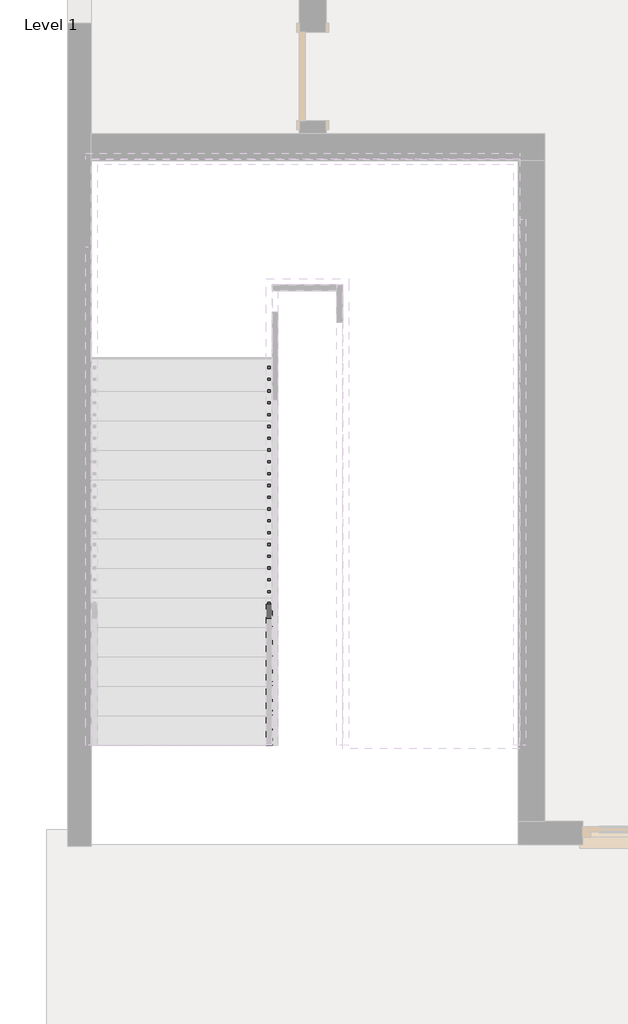
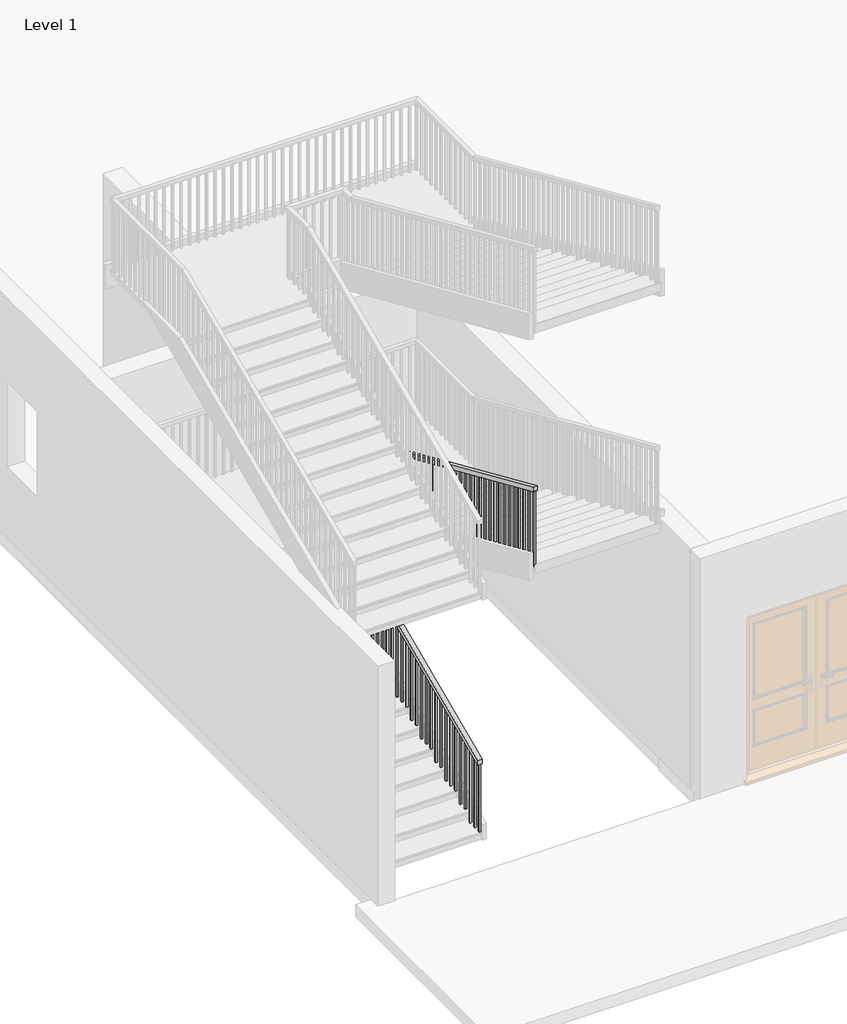
# One storey, part 2 of 6: 1 railing.
"""IFC4 building model written with IfcOpenShell, lengths in millimetres."""

from ifc_helpers import new_model, si_unit, frame, origin, place, context, project, spatial, polyline, outline, extrude, faceted_brep, element, save

model = new_model("IFC4")

# Units and contexts
model_context = context("Model", 3, world=origin())
ifc_project = project(units=[si_unit("LENGTHUNIT", "METRE", prefix="MILLI")], contexts=[model_context])

# Site, building, storey
site = spatial("IfcSite", under=ifc_project)
building = spatial("IfcBuilding", under=site)
storey = spatial("IfcBuildingStorey", under=building, Name="Level 1", Elevation=0.0)

# Railing
placement = place(None, origin())
element("IfcRailing", 1, ObjectType="Handrail - Rectangular", at=placement, inside=storey, context=model_context, shape_type="SolidModel", body=[
    faceted_brep([(-6050.7290366, -6973.0610642, 721.36), (-6050.7290366, -6973.0610642, 665.8599828), (-5999.9290366, -6973.0610642, 665.8599828), (-5999.9290366, -6973.0610642, 721.36), (-6050.7290366, -3417.0610642, 2286.0), (-6050.7290366, -3406.3792071, 2235.2), (-5999.9290366, -3406.3792071, 2235.2), (-5999.9290366, -3417.0610642, 2286.0), (-6050.7290366, -2959.8610642, 2286.0), (-6050.7290366, -2959.8610642, 2235.2), (-5999.9290366, -3010.6610642, 2235.2), (-5999.9290366, -3010.6610642, 2286.0), (-5339.5290366, -2959.8610642, 2286.0), (-5339.5290366, -2959.8610642, 2235.2), (-5390.3290366, -3010.6610642, 2235.2), (-5390.3290366, -3010.6610642, 2286.0), (-5339.5290366, -3163.0610642, 2286.0), (-5339.5290366, -3173.7429214, 2235.2), (-5390.3290366, -3173.7429214, 2235.2), (-5390.3290366, -3163.0610642, 2286.0), (-5339.5290366, -6973.0610642, 3962.4), (-5390.3290366, -6973.0610642, 3962.4), (-5390.3290366, -6973.0610642, 3906.8999828), (-5339.5290366, -6973.0610642, 3906.8999828)], [[[0, 1, 2, 3]], [[1, 0, 4, 5]], [[2, 1, 5, 6]], [[3, 2, 6, 7]], [[0, 3, 7, 4]], [[5, 4, 8, 9]], [[6, 5, 9, 10]], [[7, 6, 10, 11]], [[4, 7, 11, 8]], [[9, 8, 12, 13]], [[10, 9, 13, 14]], [[11, 10, 14, 15]], [[8, 11, 15, 12]], [[13, 12, 16, 17]], [[14, 13, 17, 18]], [[15, 14, 18, 19]], [[12, 15, 19, 16]], [[20, 21, 22, 23]], [[17, 16, 20, 23]], [[18, 17, 23, 22]], [[19, 18, 22, 21]], [[16, 19, 21, 20]]]),
    extrude(outline(polyline([(-6957.1860642, 3899.9149828), (-6938.1360642, 3891.5329828), (-6938.1360642, 2936.24), (-6957.1860642, 2936.24), (-6957.1860642, 3899.9149828)])), frame((-5374.4540366, 0.0, 0.0), z_axis=(1.0, 0.0, 0.0), x_axis=(0.0, 1.0, 0.0)), (0.0, 0.0, 1.0), 19.05),
    extrude(outline(polyline([(-6855.5860642, 3855.2109828), (-6836.5360642, 3846.8289828), (-6836.5360642, 2936.24), (-6855.5860642, 2936.24), (-6855.5860642, 3855.2109828)])), frame((-5374.4540366, 0.0, 0.0), z_axis=(1.0, 0.0, 0.0), x_axis=(0.0, 1.0, 0.0)), (0.0, 0.0, 1.0), 19.05),
    extrude(outline(polyline([(-6753.9860642, 3810.5069828), (-6734.9360642, 3802.1249828), (-6734.9360642, 2936.24), (-6753.9860642, 2936.24), (-6753.9860642, 3810.5069828)])), frame((-5374.4540366, 0.0, 0.0), z_axis=(1.0, 0.0, 0.0), x_axis=(0.0, 1.0, 0.0)), (0.0, 0.0, 1.0), 19.05),
    extrude(outline(polyline([(-6652.3860642, 3765.8029828), (-6633.3360642, 3757.4209828), (-6633.3360642, 2824.48), (-6652.3860642, 2824.48), (-6652.3860642, 3765.8029828)])), frame((-5374.4540366, 0.0, 0.0), z_axis=(1.0, 0.0, 0.0), x_axis=(0.0, 1.0, 0.0)), (0.0, 0.0, 1.0), 19.05),
    extrude(outline(polyline([(-6550.7860642, 3721.0989828), (-6531.7360642, 3712.7169828), (-6531.7360642, 2824.48), (-6550.7860642, 2824.48), (-6550.7860642, 3721.0989828)])), frame((-5374.4540366, 0.0, 0.0), z_axis=(1.0, 0.0, 0.0), x_axis=(0.0, 1.0, 0.0)), (0.0, 0.0, 1.0), 19.05),
    extrude(outline(polyline([(-6449.1860642, 3676.3949828), (-6430.1360642, 3668.0129828), (-6430.1360642, 2712.72), (-6449.1860642, 2712.72), (-6449.1860642, 3676.3949828)])), frame((-5374.4540366, 0.0, 0.0), z_axis=(1.0, 0.0, 0.0), x_axis=(0.0, 1.0, 0.0)), (0.0, 0.0, 1.0), 19.05),
    extrude(outline(polyline([(-6347.5860642, 3631.6909828), (-6328.5360642, 3623.3089828), (-6328.5360642, 2712.72), (-6347.5860642, 2712.72), (-6347.5860642, 3631.6909828)])), frame((-5374.4540366, 0.0, 0.0), z_axis=(1.0, 0.0, 0.0), x_axis=(0.0, 1.0, 0.0)), (0.0, 0.0, 1.0), 19.05),
    extrude(outline(polyline([(-6245.9860642, 3586.9869828), (-6226.9360642, 3578.6049828), (-6226.9360642, 2712.72), (-6245.9860642, 2712.72), (-6245.9860642, 3586.9869828)])), frame((-5374.4540366, 0.0, 0.0), z_axis=(1.0, 0.0, 0.0), x_axis=(0.0, 1.0, 0.0)), (0.0, 0.0, 1.0), 19.05),
    extrude(outline(polyline([(-6144.3860642, 3542.2829828), (-6125.3360642, 3533.9009828), (-6125.3360642, 2600.96), (-6144.3860642, 2600.96), (-6144.3860642, 3542.2829828)])), frame((-5374.4540366, 0.0, 0.0), z_axis=(1.0, 0.0, 0.0), x_axis=(0.0, 1.0, 0.0)), (0.0, 0.0, 1.0), 19.05),
    extrude(outline(polyline([(-6042.7860642, 3497.5789828), (-6023.7360642, 3489.1969828), (-6023.7360642, 2600.96), (-6042.7860642, 2600.96), (-6042.7860642, 3497.5789828)])), frame((-5374.4540366, 0.0, 0.0), z_axis=(1.0, 0.0, 0.0), x_axis=(0.0, 1.0, 0.0)), (0.0, 0.0, 1.0), 19.05),
    extrude(outline(polyline([(-5941.1860642, 3452.8749828), (-5922.1360642, 3444.4929828), (-5922.1360642, 2489.2), (-5941.1860642, 2489.2), (-5941.1860642, 3452.8749828)])), frame((-5374.4540366, 0.0, 0.0), z_axis=(1.0, 0.0, 0.0), x_axis=(0.0, 1.0, 0.0)), (0.0, 0.0, 1.0), 19.05),
    extrude(outline(polyline([(-5839.5860642, 3408.1709828), (-5820.5360642, 3399.7889828), (-5820.5360642, 2489.2), (-5839.5860642, 2489.2), (-5839.5860642, 3408.1709828)])), frame((-5374.4540366, 0.0, 0.0), z_axis=(1.0, 0.0, 0.0), x_axis=(0.0, 1.0, 0.0)), (0.0, 0.0, 1.0), 19.05),
    extrude(outline(polyline([(-5737.9860642, 3363.4669828), (-5718.9360642, 3355.0849828), (-5718.9360642, 2489.2), (-5737.9860642, 2489.2), (-5737.9860642, 3363.4669828)])), frame((-5374.4540366, 0.0, 0.0), z_axis=(1.0, 0.0, 0.0), x_axis=(0.0, 1.0, 0.0)), (0.0, 0.0, 1.0), 19.05),
    extrude(outline(polyline([(-5636.3860642, 3318.7629828), (-5617.3360642, 3310.3809828), (-5617.3360642, 2377.44), (-5636.3860642, 2377.44), (-5636.3860642, 3318.7629828)])), frame((-5374.4540366, 0.0, 0.0), z_axis=(1.0, 0.0, 0.0), x_axis=(0.0, 1.0, 0.0)), (0.0, 0.0, 1.0), 19.05),
    extrude(outline(polyline([(-5534.7860642, 3274.0589828), (-5515.7360642, 3265.6769828), (-5515.7360642, 2377.44), (-5534.7860642, 2377.44), (-5534.7860642, 3274.0589828)])), frame((-5374.4540366, 0.0, 0.0), z_axis=(1.0, 0.0, 0.0), x_axis=(0.0, 1.0, 0.0)), (0.0, 0.0, 1.0), 19.05),
    extrude(outline(polyline([(-5433.1860642, 3229.3549828), (-5414.1360642, 3220.9729828), (-5414.1360642, 2265.68), (-5433.1860642, 2265.68), (-5433.1860642, 3229.3549828)])), frame((-5374.4540366, 0.0, 0.0), z_axis=(1.0, 0.0, 0.0), x_axis=(0.0, 1.0, 0.0)), (0.0, 0.0, 1.0), 19.05),
    extrude(outline(polyline([(-5331.5860642, 3184.6509828), (-5312.5360642, 3176.2689828), (-5312.5360642, 2265.68), (-5331.5860642, 2265.68), (-5331.5860642, 3184.6509828)])), frame((-5374.4540366, 0.0, 0.0), z_axis=(1.0, 0.0, 0.0), x_axis=(0.0, 1.0, 0.0)), (0.0, 0.0, 1.0), 19.05),
    extrude(outline(polyline([(-5229.9860642, 3139.9469828), (-5210.9360642, 3131.5649828), (-5210.9360642, 2265.68), (-5229.9860642, 2265.68), (-5229.9860642, 3139.9469828)])), frame((-5374.4540366, 0.0, 0.0), z_axis=(1.0, 0.0, 0.0), x_axis=(0.0, 1.0, 0.0)), (0.0, 0.0, 1.0), 19.05),
    extrude(outline(polyline([(-5128.3860642, 3095.2429828), (-5109.3360642, 3086.8609828), (-5109.3360642, 2153.92), (-5128.3860642, 2153.92), (-5128.3860642, 3095.2429828)])), frame((-5374.4540366, 0.0, 0.0), z_axis=(1.0, 0.0, 0.0), x_axis=(0.0, 1.0, 0.0)), (0.0, 0.0, 1.0), 19.05),
    extrude(outline(polyline([(-5026.7860642, 3050.5389828), (-5007.7360642, 3042.1569828), (-5007.7360642, 2153.92), (-5026.7860642, 2153.92), (-5026.7860642, 3050.5389828)])), frame((-5374.4540366, 0.0, 0.0), z_axis=(1.0, 0.0, 0.0), x_axis=(0.0, 1.0, 0.0)), (0.0, 0.0, 1.0), 19.05),
    extrude(outline(polyline([(-4925.1860642, 3005.8349828), (-4906.1360642, 2997.4529828), (-4906.1360642, 2042.16), (-4925.1860642, 2042.16), (-4925.1860642, 3005.8349828)])), frame((-5374.4540366, 0.0, 0.0), z_axis=(1.0, 0.0, 0.0), x_axis=(0.0, 1.0, 0.0)), (0.0, 0.0, 1.0), 19.05),
    extrude(outline(polyline([(-4823.5860642, 2961.1309828), (-4804.5360642, 2952.7489828), (-4804.5360642, 2042.16), (-4823.5860642, 2042.16), (-4823.5860642, 2961.1309828)])), frame((-5374.4540366, 0.0, 0.0), z_axis=(1.0, 0.0, 0.0), x_axis=(0.0, 1.0, 0.0)), (0.0, 0.0, 1.0), 19.05),
    extrude(outline(polyline([(-4721.9860642, 2916.4269828), (-4702.9360642, 2908.0449828), (-4702.9360642, 2042.16), (-4721.9860642, 2042.16), (-4721.9860642, 2916.4269828)])), frame((-5374.4540366, 0.0, 0.0), z_axis=(1.0, 0.0, 0.0), x_axis=(0.0, 1.0, 0.0)), (0.0, 0.0, 1.0), 19.05),
    extrude(outline(polyline([(-4620.3860642, 2871.7229828), (-4601.3360642, 2863.3409828), (-4601.3360642, 1930.4), (-4620.3860642, 1930.4), (-4620.3860642, 2871.7229828)])), frame((-5374.4540366, 0.0, 0.0), z_axis=(1.0, 0.0, 0.0), x_axis=(0.0, 1.0, 0.0)), (0.0, 0.0, 1.0), 19.05),
    extrude(outline(polyline([(-4518.7860642, 2827.0189828), (-4499.7360642, 2818.6369828), (-4499.7360642, 1930.4), (-4518.7860642, 1930.4), (-4518.7860642, 2827.0189828)])), frame((-5374.4540366, 0.0, 0.0), z_axis=(1.0, 0.0, 0.0), x_axis=(0.0, 1.0, 0.0)), (0.0, 0.0, 1.0), 19.05),
    extrude(outline(polyline([(-4417.1860642, 2782.3149828), (-4398.1360642, 2773.9329828), (-4398.1360642, 1818.64), (-4417.1860642, 1818.64), (-4417.1860642, 2782.3149828)])), frame((-5374.4540366, 0.0, 0.0), z_axis=(1.0, 0.0, 0.0), x_axis=(0.0, 1.0, 0.0)), (0.0, 0.0, 1.0), 19.05),
    extrude(outline(polyline([(-4315.5860642, 2737.6109828), (-4296.5360642, 2729.2289828), (-4296.5360642, 1818.64), (-4315.5860642, 1818.64), (-4315.5860642, 2737.6109828)])), frame((-5374.4540366, 0.0, 0.0), z_axis=(1.0, 0.0, 0.0), x_axis=(0.0, 1.0, 0.0)), (0.0, 0.0, 1.0), 19.05),
    extrude(outline(polyline([(-4213.9860642, 2692.9069828), (-4194.9360642, 2684.5249828), (-4194.9360642, 1818.64), (-4213.9860642, 1818.64), (-4213.9860642, 2692.9069828)])), frame((-5374.4540366, 0.0, 0.0), z_axis=(1.0, 0.0, 0.0), x_axis=(0.0, 1.0, 0.0)), (0.0, 0.0, 1.0), 19.05),
    extrude(outline(polyline([(-4112.3860642, 2648.2029828), (-4093.3360642, 2639.8209828), (-4093.3360642, 1706.88), (-4112.3860642, 1706.88), (-4112.3860642, 2648.2029828)])), frame((-5374.4540366, 0.0, 0.0), z_axis=(1.0, 0.0, 0.0), x_axis=(0.0, 1.0, 0.0)), (0.0, 0.0, 1.0), 19.05),
    extrude(outline(polyline([(-4010.7860642, 2603.4989828), (-3991.7360642, 2595.1169828), (-3991.7360642, 1706.88), (-4010.7860642, 1706.88), (-4010.7860642, 2603.4989828)])), frame((-5374.4540366, 0.0, 0.0), z_axis=(1.0, 0.0, 0.0), x_axis=(0.0, 1.0, 0.0)), (0.0, 0.0, 1.0), 19.05),
    extrude(outline(polyline([(-3909.1860642, 2558.7949828), (-3890.1360642, 2550.4129828), (-3890.1360642, 1595.12), (-3909.1860642, 1595.12), (-3909.1860642, 2558.7949828)])), frame((-5374.4540366, 0.0, 0.0), z_axis=(1.0, 0.0, 0.0), x_axis=(0.0, 1.0, 0.0)), (0.0, 0.0, 1.0), 19.05),
    extrude(outline(polyline([(-3807.5860642, 2514.0909828), (-3788.5360642, 2505.7089828), (-3788.5360642, 1595.12), (-3807.5860642, 1595.12), (-3807.5860642, 2514.0909828)])), frame((-5374.4540366, 0.0, 0.0), z_axis=(1.0, 0.0, 0.0), x_axis=(0.0, 1.0, 0.0)), (0.0, 0.0, 1.0), 19.05),
    extrude(outline(polyline([(-3705.9860642, 2469.3869828), (-3686.9360642, 2461.0049828), (-3686.9360642, 1595.12), (-3705.9860642, 1595.12), (-3705.9860642, 2469.3869828)])), frame((-5374.4540366, 0.0, 0.0), z_axis=(1.0, 0.0, 0.0), x_axis=(0.0, 1.0, 0.0)), (0.0, 0.0, 1.0), 19.05),
    extrude(outline(polyline([(-3604.3860642, 2424.6829828), (-3585.3360642, 2416.3009828), (-3585.3360642, 1483.36), (-3604.3860642, 1483.36), (-3604.3860642, 2424.6829828)])), frame((-5374.4540366, 0.0, 0.0), z_axis=(1.0, 0.0, 0.0), x_axis=(0.0, 1.0, 0.0)), (0.0, 0.0, 1.0), 19.05),
    extrude(outline(polyline([(-3502.7860642, 2379.9789828), (-3483.7360642, 2371.5969828), (-3483.7360642, 1483.36), (-3502.7860642, 1483.36), (-3502.7860642, 2379.9789828)])), frame((-5374.4540366, 0.0, 0.0), z_axis=(1.0, 0.0, 0.0), x_axis=(0.0, 1.0, 0.0)), (0.0, 0.0, 1.0), 19.05),
    extrude(outline(polyline([(-3401.1860642, 2335.2749828), (-3382.1360642, 2326.8929828), (-3382.1360642, 1371.6), (-3401.1860642, 1371.6), (-3401.1860642, 2335.2749828)])), frame((-5374.4540366, 0.0, 0.0), z_axis=(1.0, 0.0, 0.0), x_axis=(0.0, 1.0, 0.0)), (0.0, 0.0, 1.0), 19.05),
    extrude(outline(polyline([(-3299.5860642, 2290.5709828), (-3280.5360642, 2282.1889828), (-3280.5360642, 1371.6), (-3299.5860642, 1371.6), (-3299.5860642, 2290.5709828)])), frame((-5374.4540366, 0.0, 0.0), z_axis=(1.0, 0.0, 0.0), x_axis=(0.0, 1.0, 0.0)), (0.0, 0.0, 1.0), 19.05),
    extrude(outline(polyline([(-3197.9860642, 2245.8669828), (-3178.9360642, 2237.4849828), (-3178.9360642, 1371.6), (-3197.9860642, 1371.6), (-3197.9860642, 2245.8669828)])), frame((-5374.4540366, 0.0, 0.0), z_axis=(1.0, 0.0, 0.0), x_axis=(0.0, 1.0, 0.0)), (0.0, 0.0, 1.0), 19.05),
    extrude(outline(polyline([(-5374.4540366, -3077.3360642), (-5355.4040366, -3077.3360642), (-5355.4040366, -3096.3860642), (-5374.4540366, -3096.3860642), (-5374.4540366, -3077.3360642)])), frame((0.0, 0.0, 1371.6), z_axis=(0.0, 0.0, 1.0), x_axis=(1.0, 0.0, 0.0)), (0.0, 0.0, 1.0), 863.6),
    extrude(outline(polyline([(-5425.2540366, -2994.7860642), (-5425.2540366, -2975.7360642), (-5406.2040366, -2975.7360642), (-5406.2040366, -2994.7860642), (-5425.2540366, -2994.7860642)])), frame((0.0, 0.0, 1371.6), z_axis=(0.0, 0.0, 1.0), x_axis=(1.0, 0.0, 0.0)), (0.0, 0.0, 1.0), 863.6),
    extrude(outline(polyline([(-5526.8540366, -2994.7860642), (-5526.8540366, -2975.7360642), (-5507.8040366, -2975.7360642), (-5507.8040366, -2994.7860642), (-5526.8540366, -2994.7860642)])), frame((0.0, 0.0, 1371.6), z_axis=(0.0, 0.0, 1.0), x_axis=(1.0, 0.0, 0.0)), (0.0, 0.0, 1.0), 863.6),
    extrude(outline(polyline([(-5628.4540366, -2994.7860642), (-5628.4540366, -2975.7360642), (-5609.4040366, -2975.7360642), (-5609.4040366, -2994.7860642), (-5628.4540366, -2994.7860642)])), frame((0.0, 0.0, 1371.6), z_axis=(0.0, 0.0, 1.0), x_axis=(1.0, 0.0, 0.0)), (0.0, 0.0, 1.0), 863.6),
    extrude(outline(polyline([(-5730.0540366, -2994.7860642), (-5730.0540366, -2975.7360642), (-5711.0040366, -2975.7360642), (-5711.0040366, -2994.7860642), (-5730.0540366, -2994.7860642)])), frame((0.0, 0.0, 1371.6), z_axis=(0.0, 0.0, 1.0), x_axis=(1.0, 0.0, 0.0)), (0.0, 0.0, 1.0), 863.6),
    extrude(outline(polyline([(-5831.6540366, -2994.7860642), (-5831.6540366, -2975.7360642), (-5812.6040366, -2975.7360642), (-5812.6040366, -2994.7860642), (-5831.6540366, -2994.7860642)])), frame((0.0, 0.0, 1371.6), z_axis=(0.0, 0.0, 1.0), x_axis=(1.0, 0.0, 0.0)), (0.0, 0.0, 1.0), 863.6),
    extrude(outline(polyline([(-5933.2540366, -2994.7860642), (-5933.2540366, -2975.7360642), (-5914.2040366, -2975.7360642), (-5914.2040366, -2994.7860642), (-5933.2540366, -2994.7860642)])), frame((0.0, 0.0, 1371.6), z_axis=(0.0, 0.0, 1.0), x_axis=(1.0, 0.0, 0.0)), (0.0, 0.0, 1.0), 863.6),
    extrude(outline(polyline([(-6015.8040366, -3020.1860642), (-6034.8540366, -3020.1860642), (-6034.8540366, -3001.1360642), (-6015.8040366, -3001.1360642), (-6015.8040366, -3020.1860642)])), frame((0.0, 0.0, 1371.6), z_axis=(0.0, 0.0, 1.0), x_axis=(1.0, 0.0, 0.0)), (0.0, 0.0, 1.0), 863.6),
    extrude(outline(polyline([(-6015.8040366, -3121.7860642), (-6034.8540366, -3121.7860642), (-6034.8540366, -3102.7360642), (-6015.8040366, -3102.7360642), (-6015.8040366, -3121.7860642)])), frame((0.0, 0.0, 1371.6), z_axis=(0.0, 0.0, 1.0), x_axis=(1.0, 0.0, 0.0)), (0.0, 0.0, 1.0), 863.6),
    extrude(outline(polyline([(-6015.8040366, -3223.3860642), (-6034.8540366, -3223.3860642), (-6034.8540366, -3204.3360642), (-6015.8040366, -3204.3360642), (-6015.8040366, -3223.3860642)])), frame((0.0, 0.0, 1371.6), z_axis=(0.0, 0.0, 1.0), x_axis=(1.0, 0.0, 0.0)), (0.0, 0.0, 1.0), 863.6),
    extrude(outline(polyline([(-6015.8040366, -3324.9860642), (-6034.8540366, -3324.9860642), (-6034.8540366, -3305.9360642), (-6015.8040366, -3305.9360642), (-6015.8040366, -3324.9860642)])), frame((0.0, 0.0, 1371.6), z_axis=(0.0, 0.0, 1.0), x_axis=(1.0, 0.0, 0.0)), (0.0, 0.0, 1.0), 863.6),
    extrude(outline(polyline([(-3426.5860642, 2226.3089828), (-3407.5360642, 2234.6909828), (-3407.5360642, 1371.6), (-3426.5860642, 1371.6), (-3426.5860642, 2226.3089828)])), frame((-6034.8540366, 0.0, 0.0), z_axis=(1.0, 0.0, 0.0), x_axis=(0.0, 1.0, 0.0)), (0.0, 0.0, 1.0), 19.05),
    extrude(outline(polyline([(-3528.1860642, 2181.6049828), (-3509.1360642, 2189.9869828), (-3509.1360642, 1259.84), (-3528.1860642, 1259.84), (-3528.1860642, 2181.6049828)])), frame((-6034.8540366, 0.0, 0.0), z_axis=(1.0, 0.0, 0.0), x_axis=(0.0, 1.0, 0.0)), (0.0, 0.0, 1.0), 19.05),
    extrude(outline(polyline([(-3629.7860642, 2136.9009828), (-3610.7360642, 2145.2829828), (-3610.7360642, 1259.84), (-3629.7860642, 1259.84), (-3629.7860642, 2136.9009828)])), frame((-6034.8540366, 0.0, 0.0), z_axis=(1.0, 0.0, 0.0), x_axis=(0.0, 1.0, 0.0)), (0.0, 0.0, 1.0), 19.05),
    extrude(outline(polyline([(-3731.3860642, 2092.1969828), (-3712.3360642, 2100.5789828), (-3712.3360642, 1148.08), (-3731.3860642, 1148.08), (-3731.3860642, 2092.1969828)])), frame((-6034.8540366, 0.0, 0.0), z_axis=(1.0, 0.0, 0.0), x_axis=(0.0, 1.0, 0.0)), (0.0, 0.0, 1.0), 19.05),
    extrude(outline(polyline([(-3832.9860642, 2047.4929828), (-3813.9360642, 2055.8749828), (-3813.9360642, 1148.08), (-3832.9860642, 1148.08), (-3832.9860642, 2047.4929828)])), frame((-6034.8540366, 0.0, 0.0), z_axis=(1.0, 0.0, 0.0), x_axis=(0.0, 1.0, 0.0)), (0.0, 0.0, 1.0), 19.05),
    extrude(outline(polyline([(-3934.5860642, 2002.7889828), (-3915.5360642, 2011.1709828), (-3915.5360642, 1148.08), (-3934.5860642, 1148.08), (-3934.5860642, 2002.7889828)])), frame((-6034.8540366, 0.0, 0.0), z_axis=(1.0, 0.0, 0.0), x_axis=(0.0, 1.0, 0.0)), (0.0, 0.0, 1.0), 19.05),
    extrude(outline(polyline([(-4036.1860642, 1958.0849828), (-4017.1360642, 1966.4669828), (-4017.1360642, 1036.32), (-4036.1860642, 1036.32), (-4036.1860642, 1958.0849828)])), frame((-6034.8540366, 0.0, 0.0), z_axis=(1.0, 0.0, 0.0), x_axis=(0.0, 1.0, 0.0)), (0.0, 0.0, 1.0), 19.05),
    extrude(outline(polyline([(-4137.7860642, 1913.3809828), (-4118.7360642, 1921.7629828), (-4118.7360642, 1036.32), (-4137.7860642, 1036.32), (-4137.7860642, 1913.3809828)])), frame((-6034.8540366, 0.0, 0.0), z_axis=(1.0, 0.0, 0.0), x_axis=(0.0, 1.0, 0.0)), (0.0, 0.0, 1.0), 19.05),
    extrude(outline(polyline([(-4239.3860642, 1868.6769828), (-4220.3360642, 1877.0589828), (-4220.3360642, 924.56), (-4239.3860642, 924.56), (-4239.3860642, 1868.6769828)])), frame((-6034.8540366, 0.0, 0.0), z_axis=(1.0, 0.0, 0.0), x_axis=(0.0, 1.0, 0.0)), (0.0, 0.0, 1.0), 19.05),
    extrude(outline(polyline([(-4340.9860642, 1823.9729828), (-4321.9360642, 1832.3549828), (-4321.9360642, 924.56), (-4340.9860642, 924.56), (-4340.9860642, 1823.9729828)])), frame((-6034.8540366, 0.0, 0.0), z_axis=(1.0, 0.0, 0.0), x_axis=(0.0, 1.0, 0.0)), (0.0, 0.0, 1.0), 19.05),
    extrude(outline(polyline([(-4442.5860642, 1779.2689828), (-4423.5360642, 1787.6509828), (-4423.5360642, 924.56), (-4442.5860642, 924.56), (-4442.5860642, 1779.2689828)])), frame((-6034.8540366, 0.0, 0.0), z_axis=(1.0, 0.0, 0.0), x_axis=(0.0, 1.0, 0.0)), (0.0, 0.0, 1.0), 19.05),
    extrude(outline(polyline([(-4544.1860642, 1734.5649828), (-4525.1360642, 1742.9469828), (-4525.1360642, 812.8), (-4544.1860642, 812.8), (-4544.1860642, 1734.5649828)])), frame((-6034.8540366, 0.0, 0.0), z_axis=(1.0, 0.0, 0.0), x_axis=(0.0, 1.0, 0.0)), (0.0, 0.0, 1.0), 19.05),
    extrude(outline(polyline([(-4645.7860642, 1689.8609828), (-4626.7360642, 1698.2429828), (-4626.7360642, 812.8), (-4645.7860642, 812.8), (-4645.7860642, 1689.8609828)])), frame((-6034.8540366, 0.0, 0.0), z_axis=(1.0, 0.0, 0.0), x_axis=(0.0, 1.0, 0.0)), (0.0, 0.0, 1.0), 19.05),
    extrude(outline(polyline([(-4747.3860642, 1645.1569828), (-4728.3360642, 1653.5389828), (-4728.3360642, 701.04), (-4747.3860642, 701.04), (-4747.3860642, 1645.1569828)])), frame((-6034.8540366, 0.0, 0.0), z_axis=(1.0, 0.0, 0.0), x_axis=(0.0, 1.0, 0.0)), (0.0, 0.0, 1.0), 19.05),
    extrude(outline(polyline([(-4848.9860642, 1600.4529828), (-4829.9360642, 1608.8349828), (-4829.9360642, 701.04), (-4848.9860642, 701.04), (-4848.9860642, 1600.4529828)])), frame((-6034.8540366, 0.0, 0.0), z_axis=(1.0, 0.0, 0.0), x_axis=(0.0, 1.0, 0.0)), (0.0, 0.0, 1.0), 19.05),
    extrude(outline(polyline([(-4950.5860642, 1555.7489828), (-4931.5360642, 1564.1309828), (-4931.5360642, 701.04), (-4950.5860642, 701.04), (-4950.5860642, 1555.7489828)])), frame((-6034.8540366, 0.0, 0.0), z_axis=(1.0, 0.0, 0.0), x_axis=(0.0, 1.0, 0.0)), (0.0, 0.0, 1.0), 19.05),
    extrude(outline(polyline([(-5052.1860642, 1511.0449828), (-5033.1360642, 1519.4269828), (-5033.1360642, 589.28), (-5052.1860642, 589.28), (-5052.1860642, 1511.0449828)])), frame((-6034.8540366, 0.0, 0.0), z_axis=(1.0, 0.0, 0.0), x_axis=(0.0, 1.0, 0.0)), (0.0, 0.0, 1.0), 19.05),
    extrude(outline(polyline([(-5153.7860642, 1466.3409828), (-5134.7360642, 1474.7229828), (-5134.7360642, 589.28), (-5153.7860642, 589.28), (-5153.7860642, 1466.3409828)])), frame((-6034.8540366, 0.0, 0.0), z_axis=(1.0, 0.0, 0.0), x_axis=(0.0, 1.0, 0.0)), (0.0, 0.0, 1.0), 19.05),
    extrude(outline(polyline([(-5255.3860642, 1421.6369828), (-5236.3360642, 1430.0189828), (-5236.3360642, 477.52), (-5255.3860642, 477.52), (-5255.3860642, 1421.6369828)])), frame((-6034.8540366, 0.0, 0.0), z_axis=(1.0, 0.0, 0.0), x_axis=(0.0, 1.0, 0.0)), (0.0, 0.0, 1.0), 19.05),
    extrude(outline(polyline([(-5356.9860642, 1376.9329828), (-5337.9360642, 1385.3149828), (-5337.9360642, 477.52), (-5356.9860642, 477.52), (-5356.9860642, 1376.9329828)])), frame((-6034.8540366, 0.0, 0.0), z_axis=(1.0, 0.0, 0.0), x_axis=(0.0, 1.0, 0.0)), (0.0, 0.0, 1.0), 19.05),
    extrude(outline(polyline([(-5458.5860642, 1332.2289828), (-5439.5360642, 1340.6109828), (-5439.5360642, 477.52), (-5458.5860642, 477.52), (-5458.5860642, 1332.2289828)])), frame((-6034.8540366, 0.0, 0.0), z_axis=(1.0, 0.0, 0.0), x_axis=(0.0, 1.0, 0.0)), (0.0, 0.0, 1.0), 19.05),
    extrude(outline(polyline([(-5560.1860642, 1287.5249828), (-5541.1360642, 1295.9069828), (-5541.1360642, 365.76), (-5560.1860642, 365.76), (-5560.1860642, 1287.5249828)])), frame((-6034.8540366, 0.0, 0.0), z_axis=(1.0, 0.0, 0.0), x_axis=(0.0, 1.0, 0.0)), (0.0, 0.0, 1.0), 19.05),
    extrude(outline(polyline([(-5661.7860642, 1242.8209828), (-5642.7360642, 1251.2029828), (-5642.7360642, 365.76), (-5661.7860642, 365.76), (-5661.7860642, 1242.8209828)])), frame((-6034.8540366, 0.0, 0.0), z_axis=(1.0, 0.0, 0.0), x_axis=(0.0, 1.0, 0.0)), (0.0, 0.0, 1.0), 19.05),
    extrude(outline(polyline([(-5763.3860642, 1198.1169828), (-5744.3360642, 1206.4989828), (-5744.3360642, 254.0), (-5763.3860642, 254.0), (-5763.3860642, 1198.1169828)])), frame((-6034.8540366, 0.0, 0.0), z_axis=(1.0, 0.0, 0.0), x_axis=(0.0, 1.0, 0.0)), (0.0, 0.0, 1.0), 19.05),
    extrude(outline(polyline([(-5864.9860642, 1153.4129828), (-5845.9360642, 1161.7949828), (-5845.9360642, 254.0), (-5864.9860642, 254.0), (-5864.9860642, 1153.4129828)])), frame((-6034.8540366, 0.0, 0.0), z_axis=(1.0, 0.0, 0.0), x_axis=(0.0, 1.0, 0.0)), (0.0, 0.0, 1.0), 19.05),
    extrude(outline(polyline([(-5966.5860642, 1108.7089828), (-5947.5360642, 1117.0909828), (-5947.5360642, 254.0), (-5966.5860642, 254.0), (-5966.5860642, 1108.7089828)])), frame((-6034.8540366, 0.0, 0.0), z_axis=(1.0, 0.0, 0.0), x_axis=(0.0, 1.0, 0.0)), (0.0, 0.0, 1.0), 19.05),
    extrude(outline(polyline([(-6068.1860642, 1064.0049828), (-6049.1360642, 1072.3869828), (-6049.1360642, 142.24), (-6068.1860642, 142.24), (-6068.1860642, 1064.0049828)])), frame((-6034.8540366, 0.0, 0.0), z_axis=(1.0, 0.0, 0.0), x_axis=(0.0, 1.0, 0.0)), (0.0, 0.0, 1.0), 19.05),
    extrude(outline(polyline([(-6169.7860642, 1019.3009828), (-6150.7360642, 1027.6829828), (-6150.7360642, 142.24), (-6169.7860642, 142.24), (-6169.7860642, 1019.3009828)])), frame((-6034.8540366, 0.0, 0.0), z_axis=(1.0, 0.0, 0.0), x_axis=(0.0, 1.0, 0.0)), (0.0, 0.0, 1.0), 19.05),
    extrude(outline(polyline([(-6271.3860642, 974.5969828), (-6252.3360642, 982.9789828), (-6252.3360642, 30.48), (-6271.3860642, 30.48), (-6271.3860642, 974.5969828)])), frame((-6034.8540366, 0.0, 0.0), z_axis=(1.0, 0.0, 0.0), x_axis=(0.0, 1.0, 0.0)), (0.0, 0.0, 1.0), 19.05),
    extrude(outline(polyline([(-6372.9860642, 929.8929828), (-6353.9360642, 938.2749828), (-6353.9360642, 30.48), (-6372.9860642, 30.48), (-6372.9860642, 929.8929828)])), frame((-6034.8540366, 0.0, 0.0), z_axis=(1.0, 0.0, 0.0), x_axis=(0.0, 1.0, 0.0)), (0.0, 0.0, 1.0), 19.05),
    extrude(outline(polyline([(-6474.5860642, 885.1889828), (-6455.5360642, 893.5709828), (-6455.5360642, 30.48), (-6474.5860642, 30.48), (-6474.5860642, 885.1889828)])), frame((-6034.8540366, 0.0, 0.0), z_axis=(1.0, 0.0, 0.0), x_axis=(0.0, 1.0, 0.0)), (0.0, 0.0, 1.0), 19.05),
    extrude(outline(polyline([(-6576.1860642, 840.4849828), (-6557.1360642, 848.8669828), (-6557.1360642, -81.28), (-6576.1860642, -81.28), (-6576.1860642, 840.4849828)])), frame((-6034.8540366, 0.0, 0.0), z_axis=(1.0, 0.0, 0.0), x_axis=(0.0, 1.0, 0.0)), (0.0, 0.0, 1.0), 19.05),
    extrude(outline(polyline([(-6677.7860642, 795.7809828), (-6658.7360642, 804.1629828), (-6658.7360642, -81.28), (-6677.7860642, -81.28), (-6677.7860642, 795.7809828)])), frame((-6034.8540366, 0.0, 0.0), z_axis=(1.0, 0.0, 0.0), x_axis=(0.0, 1.0, 0.0)), (0.0, 0.0, 1.0), 19.05),
    extrude(outline(polyline([(-6779.3860642, 751.0769828), (-6760.3360642, 759.4589828), (-6760.3360642, -193.04), (-6779.3860642, -193.04), (-6779.3860642, 751.0769828)])), frame((-6034.8540366, 0.0, 0.0), z_axis=(1.0, 0.0, 0.0), x_axis=(0.0, 1.0, 0.0)), (0.0, 0.0, 1.0), 19.05),
    extrude(outline(polyline([(-6880.9860642, 706.3729828), (-6861.9360642, 714.7549828), (-6861.9360642, -193.04), (-6880.9860642, -193.04), (-6880.9860642, 706.3729828)])), frame((-6034.8540366, 0.0, 0.0), z_axis=(1.0, 0.0, 0.0), x_axis=(0.0, 1.0, 0.0)), (0.0, 0.0, 1.0), 19.05),
    extrude(outline(polyline([(-5374.4540366, -2994.7860642), (-5374.4540366, -2975.7360642), (-5355.4040366, -2975.7360642), (-5355.4040366, -2994.7860642), (-5374.4540366, -2994.7860642)])), frame((0.0, 0.0, 1371.6), z_axis=(0.0, 0.0, 1.0), x_axis=(1.0, 0.0, 0.0)), (0.0, 0.0, 1.0), 863.6),
    extrude(outline(polyline([(-6015.8040366, -2994.7860642), (-6034.8540366, -2994.7860642), (-6034.8540366, -2975.7360642), (-6015.8040366, -2975.7360642), (-6015.8040366, -2994.7860642)])), frame((0.0, 0.0, 1371.6), z_axis=(0.0, 0.0, 1.0), x_axis=(1.0, 0.0, 0.0)), (0.0, 0.0, 1.0), 863.6),
    extrude(outline(polyline([(-6973.0610642, 3906.8999828), (-6954.0110642, 3898.5179828), (-6954.0110642, 2936.24), (-6973.0610642, 2936.24), (-6973.0610642, 3906.8999828)])), frame((-5374.4540366, 0.0, 0.0), z_axis=(1.0, 0.0, 0.0), x_axis=(0.0, 1.0, 0.0)), (0.0, 0.0, 1.0), 19.05),
    extrude(outline(polyline([(-6973.0610642, 665.8599828), (-6954.0110642, 674.2419828), (-6954.0110642, -193.04), (-6973.0610642, -193.04), (-6973.0610642, 665.8599828)])), frame((-6034.8540366, 0.0, 0.0), z_axis=(1.0, 0.0, 0.0), x_axis=(0.0, 1.0, 0.0)), (0.0, 0.0, 1.0), 19.05),
])

save(model, "model.ifc")

# Revit data of these elements
# Type "Handrail - Rectangular"
#   Assembly Code = "C2010400"
#   built-in parameter 1008612 = 0.0416667 (stored number, unit not read)
#   built-in parameter 1008611 = 0.0416667 (stored number, unit not read)
#   built-in parameter 1008609 = 0.333333 (stored number, unit not read)
#   built-in parameter 1008604 = 0.166667 (stored number, unit not read)
#   built-in parameter 1008603 = 0.166667 (stored number, unit not read)
#   Railing Height = 3' - 0"
#   built-in parameter 1008630 = 2
#   built-in parameter 1008610 = 2
#   built-in parameter 1008618 = Baluster - Square : 3/4"
# Element 1 (IfcRailing, "Handrail - Rectangular")
#   Phase Created = New Construction
